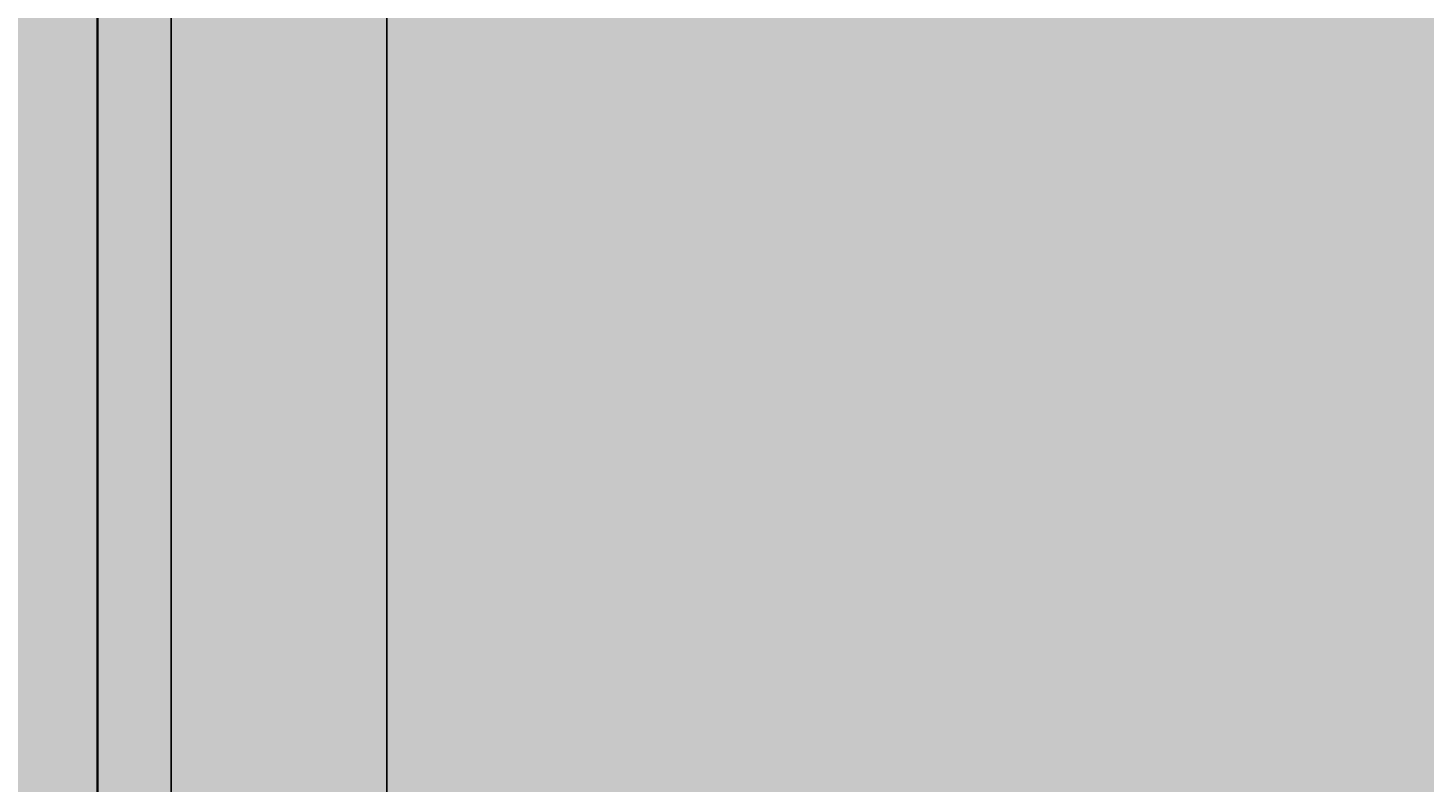
# Model space of a CAD drawing. Units: feet. Extents: x 2695 to 2912, y 795 to 1139.
# Tile 69 of 83: x 2769 to 2805, y 1081 to 1100. Entities that reach past the tile are written whole.
import ezdxf

# ---------------------------------------------------------------- set-up
doc = ezdxf.new("R2010")
doc.units = ezdxf.units.FT
for name, color, linetype, lineweight in [('A-ANNO-DIMS', 2, 'Continuous', 18), ('A-ELEV', 7, 'Continuous', 35), ('A-ELEV-PATT', 252, 'Continuous', 13)]:
    doc.layers.add(name, color=color, linetype=linetype, lineweight=lineweight)
doc.styles.get("Standard").update_dxf_attribs({"font": 'arial.ttf'})
doc.dimstyles.get("Standard").update_dxf_attribs({"dimtxt": 0.18, "dimasz": 0.18, "dimexe": 0.18, "dimexo": 0.0625, "dimgap": 0.09, "dimtad": 0, "dimtih": 1, "dimtoh": 1, "dimdec": 1, "dimzin": 0, "dimdsep": 46, "dimlunit": 3, "dimtxsty": 'Standard', "dimcen": 0.09, "dimadec": 0, "dimazin": 0, "dimtfac": 1, "dimtdec": 1, "dimtofl": 0, "dimtmove": 0, "dimatfit": 3, "dimfxl": 1, "dimtolj": 1, "dimtzin": 0, "dimarcsym": 0})

# ---------------------------------------------------------------- blocks, each defined once
blk = doc.blocks.new('*D8')
at = {"layer": 'A-ANNO-DIMS', "color": 0, "lineweight": -2, "transparency": 16777216}
for p, q in [((2715.885, 1050.373), (2715.885, 1138.886)), ((2716.065, 1138.706), (2742.866, 1138.706)), ((2770.456, 1138.706), (2743.655, 1138.706)), ((2770.636, 1122.993), (2770.636, 1138.886))]:
    blk.add_line(p, q, dxfattribs=at)
at = {"layer": 'A-ANNO-DIMS', "color": 0, "transparency": 16777216}
for points in [[(2716.065, 1138.736), (2716.065, 1138.676), (2715.885, 1138.706)], [(2770.456, 1138.736), (2770.456, 1138.676), (2770.636, 1138.706)]]:
    blk.add_solid(points, dxfattribs=at)
at = {"layer": 'Defpoints', "color": 0, "transparency": 16777216}
for p in [(2770.636, 1138.706), (2770.636, 1122.931), (2715.885, 1050.311)]:
    blk.add_point(p, dxfattribs=at)
at = {"layer": 'A-ANNO-DIMS', "color": 0, "transparency": 16777216, "insert": (2743.261, 1138.706), "char_height": 0.18, "attachment_point": 5}
blk.add_mtext('\\A1;54.75', dxfattribs=at)
blk = doc.blocks.new('*D9')
at = {"layer": 'A-ANNO-DIMS', "color": 0, "lineweight": -2, "transparency": 16777216}
for p, q in [((2770.636, 1122.993), (2770.636, 1138.886)), ((2770.816, 1138.706), (2773.942, 1138.706)), ((2777.854, 1138.706), (2774.728, 1138.706)), ((2778.034, 1020.886), (2778.034, 1138.886))]:
    blk.add_line(p, q, dxfattribs=at)
at = {"layer": 'A-ANNO-DIMS', "color": 0, "transparency": 16777216}
for points in [[(2770.816, 1138.736), (2770.816, 1138.676), (2770.636, 1138.706)], [(2777.854, 1138.736), (2777.854, 1138.676), (2778.034, 1138.706)]]:
    blk.add_solid(points, dxfattribs=at)
at = {"layer": 'Defpoints', "color": 0, "transparency": 16777216}
for p in [(2778.034, 1138.706), (2770.636, 1122.931), (2778.034, 1020.824)]:
    blk.add_point(p, dxfattribs=at)
at = {"layer": 'A-ANNO-DIMS', "color": 0, "transparency": 16777216, "insert": (2774.335, 1138.706), "char_height": 0.18, "attachment_point": 5}
blk.add_mtext('\\A1;7.398', dxfattribs=at)
blk = doc.blocks.new('*D10')
at = {"layer": 'A-ANNO-DIMS', "color": 0, "lineweight": -2, "transparency": 16777216}
for p, q in [((2778.034, 1020.886), (2778.034, 1138.886)), ((2778.214, 1138.706), (2810.411, 1138.706)), ((2843.395, 1138.706), (2811.198, 1138.706)), ((2843.575, 1020.886), (2843.575, 1138.886))]:
    blk.add_line(p, q, dxfattribs=at)
at = {"layer": 'A-ANNO-DIMS', "color": 0, "transparency": 16777216}
for points in [[(2778.214, 1138.736), (2778.214, 1138.676), (2778.034, 1138.706)], [(2843.395, 1138.736), (2843.395, 1138.676), (2843.575, 1138.706)]]:
    blk.add_solid(points, dxfattribs=at)
at = {"layer": 'Defpoints', "color": 0, "transparency": 16777216}
for p in [(2843.575, 1138.706), (2778.034, 1020.824), (2843.575, 1020.824)]:
    blk.add_point(p, dxfattribs=at)
at = {"layer": 'A-ANNO-DIMS', "color": 0, "transparency": 16777216, "insert": (2810.805, 1138.706), "char_height": 0.18, "attachment_point": 5}
blk.add_mtext('\\A1;65.54', dxfattribs=at)
blk = doc.blocks.new('*D48')
at = {"layer": 'A-ANNO-DIMS', "color": 0, "lineweight": -2, "transparency": 16777216}
for p, q in [((2770.636, 972.03), (2770.636, 1138.886)), ((2770.816, 1138.706), (2771.263, 1138.706)), ((2772.342, 1138.706), (2771.894, 1138.706)), ((2772.522, 972.03), (2772.522, 1138.886))]:
    blk.add_line(p, q, dxfattribs=at)
at = {"layer": 'A-ANNO-DIMS', "color": 0, "transparency": 16777216}
for points in [[(2770.816, 1138.736), (2770.816, 1138.676), (2770.636, 1138.706)], [(2772.342, 1138.736), (2772.342, 1138.676), (2772.522, 1138.706)]]:
    blk.add_solid(points, dxfattribs=at)
at = {"layer": 'Defpoints', "color": 0, "transparency": 16777216}
for p in [(2772.522, 1138.706), (2770.636, 971.967), (2772.522, 971.967)]:
    blk.add_point(p, dxfattribs=at)
at = {"layer": 'A-ANNO-DIMS', "color": 0, "transparency": 16777216, "insert": (2771.579, 1138.706), "char_height": 0.18, "attachment_point": 5}
blk.add_mtext('\\A1;1.89', dxfattribs=at)
blk = doc.blocks.new('*D49')
at = {"layer": 'A-ANNO-DIMS', "color": 0, "lineweight": -2, "transparency": 16777216}
for p, q in [((2772.522, 972.03), (2772.522, 1138.886)), ((2772.702, 1138.706), (2790.888, 1138.706)), ((2809.861, 1138.706), (2791.674, 1138.706)), ((2810.041, 972.03), (2810.041, 1138.886))]:
    blk.add_line(p, q, dxfattribs=at)
at = {"layer": 'A-ANNO-DIMS', "color": 0, "transparency": 16777216}
for points in [[(2772.702, 1138.736), (2772.702, 1138.676), (2772.522, 1138.706)], [(2809.861, 1138.736), (2809.861, 1138.676), (2810.041, 1138.706)]]:
    blk.add_solid(points, dxfattribs=at)
at = {"layer": 'Defpoints', "color": 0, "transparency": 16777216}
for p in [(2810.041, 1138.706), (2772.522, 971.967), (2810.041, 971.967)]:
    blk.add_point(p, dxfattribs=at)
at = {"layer": 'A-ANNO-DIMS', "color": 0, "transparency": 16777216, "insert": (2791.281, 1138.706), "char_height": 0.18, "attachment_point": 5}
blk.add_mtext('\\A1;37.52', dxfattribs=at)

msp = doc.modelspace()

# ---------------------------------------------------------------- hatches: boundary and pattern name
at = {"layer": 'A-ELEV-PATT'}
h = msp.add_hatch(color=256, dxfattribs=at)
h.set_gradient(color1=(147, 149, 152), color2=(147, 149, 152), tint=1)
h.paths.add_polyline_path([(2770.6361, 1118.4096), (2710.6361, 1118.4096), (2710.6361, 1062.9306), (2770.6361, 1062.9306)])
h.paths.add_polyline_path([(2890.6361, 1103.3378), (2770.6361, 1103.3378), (2770.6361, 1062.9306), (2890.6361, 1062.9306)])
h.paths.add_polyline_path([(2730.7081, 1048.1052), (2755.1125, 1048.1052), (2755.1125, 936.9306), (2770.6361, 936.9306), (2770.6361, 1050.3105), (2715.8852, 1050.3105), (2715.8852, 936.9306), (2730.7081, 936.9306)])
h.paths.add_polyline_path([(2890.6361, 1050.3105), (2770.6361, 1050.3105), (2770.6361, 971.9673), (2778.0341, 971.9673), (2778.0341, 1020.8235), (2843.575, 1020.8235), (2843.575, 971.9673), (2890.6361, 971.9673)])
h.paths.add_polyline_path([(2888.1882, 970.7156), (2843.575, 970.7156), (2843.575, 964.8267), (2888.1882, 964.8267)])
h.paths.add_polyline_path([(2888.1882, 964.1328), (2843.575, 964.1328), (2843.575, 956.614), (2888.1882, 956.614)])
h.paths.add_polyline_path([(2888.1882, 955.9202), (2843.575, 955.9202), (2843.575, 949.2892), (2888.1882, 949.2892)])
h.paths.add_polyline_path([(2888.1882, 948.5954), (2843.575, 948.5954), (2843.575, 941.3507), (2888.1882, 941.3507)])
h.paths.add_polyline_path([(2888.1882, 940.6569), (2843.575, 940.6569), (2843.575, 936.9306), (2888.1882, 936.9306)])
h.paths.add_polyline_path([(2890.6361, 970.7156), (2888.9368, 970.7156), (2888.9368, 964.8267), (2890.6361, 964.8267)])
h.paths.add_polyline_path([(2890.6361, 964.1328), (2888.9368, 964.1328), (2888.9368, 956.614), (2890.6361, 956.614)])
h.paths.add_polyline_path([(2890.6361, 955.9202), (2888.9368, 955.9202), (2888.9368, 949.2892), (2890.6361, 949.2892)])
h.paths.add_polyline_path([(2890.6361, 940.6569), (2888.9368, 940.6569), (2888.9368, 936.9306), (2890.6361, 936.9306)])
h.paths.add_polyline_path([(2890.6361, 948.5954), (2888.9368, 948.5954), (2888.9368, 941.3507), (2890.6361, 941.3507)])
h.paths.add_polyline_path([(2772.5216, 970.7156), (2770.6361, 970.7156), (2770.6361, 964.8267), (2772.5216, 964.8267)])
h.paths.add_polyline_path([(2772.5216, 964.1328), (2770.6361, 964.1328), (2770.6361, 956.614), (2772.5216, 956.614)])
h.paths.add_polyline_path([(2772.5216, 955.9202), (2770.6361, 955.9202), (2770.6361, 949.2892), (2772.5216, 949.2892)])
h.paths.add_polyline_path([(2772.5216, 948.5954), (2770.6361, 948.5954), (2770.6361, 941.3507), (2772.5216, 941.3507)])
h.paths.add_polyline_path([(2772.5216, 940.6569), (2770.6361, 940.6569), (2770.6361, 936.9306), (2772.5216, 936.9306)])
h.paths.add_polyline_path([(2778.0341, 940.6569), (2773.2702, 940.6569), (2773.2702, 936.9306), (2778.0341, 936.9306)])
h.paths.add_polyline_path([(2778.0341, 970.7156), (2773.2702, 970.7156), (2773.2702, 964.8267), (2778.0341, 964.8267)])
h.paths.add_polyline_path([(2778.0341, 964.1328), (2773.2702, 964.1328), (2773.2702, 956.614), (2778.0341, 956.614)])
h.paths.add_polyline_path([(2778.0341, 955.9202), (2773.2702, 955.9202), (2773.2702, 949.2892), (2778.0341, 949.2892)])
h.paths.add_polyline_path([(2778.0341, 948.5954), (2773.2702, 948.5954), (2773.2702, 941.3507), (2778.0341, 941.3507)])
h.paths.add_polyline_path([(2810.0407, 940.6569), (2780.0341, 940.6569), (2780.0341, 936.9306), (2810.0407, 936.9306)])
h.paths.add_polyline_path([(2890.6361, 924.3105), (2770.6361, 924.3105), (2770.6361, 810.9306), (2773.5029, 810.9306), (2773.5029, 905.5143), (2805.9398, 905.5143), (2838.3767, 905.5143), (2838.3767, 810.9306), (2890.6361, 810.9306)])
h = msp.add_hatch(color=256, dxfattribs=at)
h.set_gradient(color1=(199, 200, 202), color2=(213, 227, 240), centered=1)
h.paths.add_polyline_path([(2890.6361, 1103.3378), (2770.6361, 1103.3378), (2770.6361, 1062.9306), (2890.6361, 1062.9306)])

# ---------------------------------------------------------------- linework, layer by layer
at = {"layer": 'A-ELEV'}
msp.add_line((2770.6361, 1122.9306), (2770.6361, 1062.9306), dxfattribs=at)

# ---------------------------------------------------------------- dimensions: what is measured, and where the dimension line sits
at = {"layer": 'A-ANNO-DIMS'}
for base, p1, p2, override, picture, middle in [((2770.6361, 1138.7056), (2715.8852, 1050.3105), (2770.6361, 1122.9306), {"dimdec": 2, "dimlfac": 1, "dimrnd": 0, "dimzin": 0, "dimdsep": 46, "dimlunit": 2}, '*D8', (2743.2606, 1138.7056)), ((2778.0341, 1138.7056), (2770.6361, 1122.9306), (2778.0341, 1020.8235), {"dimdec": 3, "dimlfac": 1, "dimrnd": 0, "dimzin": 0, "dimdsep": 46, "dimlunit": 2}, '*D9', (2774.3351, 1138.7056)), ((2772.5216, 1138.7056), (2770.6361, 971.9673), (2772.5216, 971.9673), {"dimdec": 2, "dimlfac": 1, "dimrnd": 0, "dimzin": 0, "dimdsep": 46, "dimlunit": 2}, '*D48', (2771.5788, 1138.7056)), ((2810.0407, 1138.7056), (2772.5216, 971.9673), (2810.0407, 971.9673), {"dimdec": 2, "dimlfac": 1, "dimrnd": 0, "dimzin": 0, "dimdsep": 46, "dimlunit": 2}, '*D49', (2791.2811, 1138.7056)), ((2843.575, 1138.7056), (2778.0341, 1020.8235), (2843.575, 1020.8235), {"dimdec": 2, "dimlfac": 1, "dimrnd": 0, "dimzin": 0, "dimdsep": 46, "dimlunit": 2}, '*D10', (2810.8045, 1138.7056))]:
    dim = msp.add_linear_dim(base=base, p1=p1, p2=p2, dimstyle='Standard', override=override, dxfattribs=at)
    dim.commit()
    dim.dimension.update_dxf_attribs({"geometry": picture, "text_midpoint": middle})

doc.saveas('drawing.dxf')
